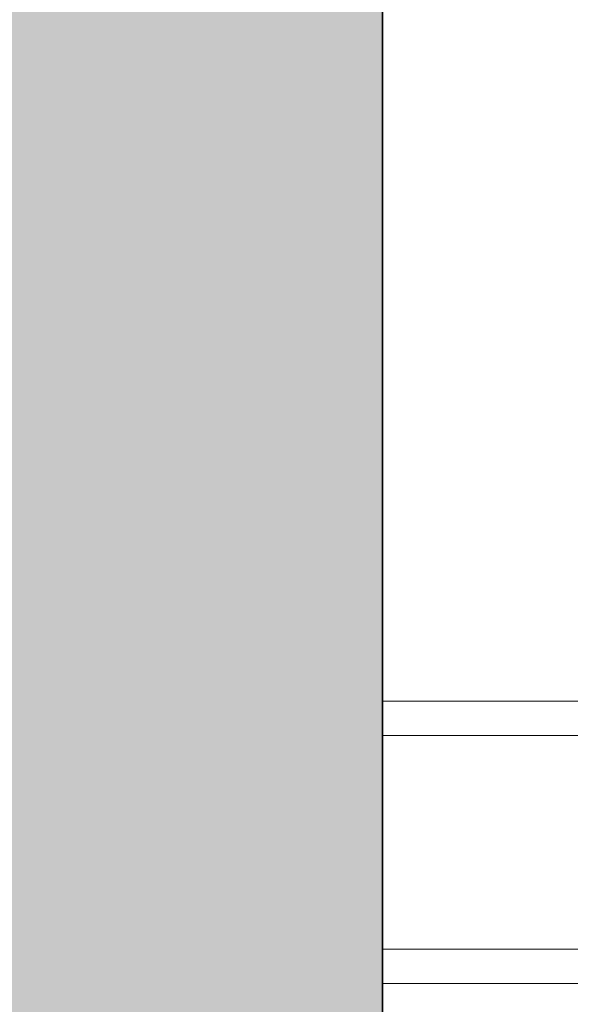
# Model space of a CAD drawing. Units: inches. Extents: x 2696 to 3240, y 1564 to 2310.
# Tile 8 of 76: x 2893.424 to 2898.411, y 1643.56 to 1652.487. Entities that reach past the tile are written whole.
import ezdxf

# ---------------------------------------------------------------- set-up
doc = ezdxf.new("R2010")
doc.units = ezdxf.units.IN
for name, color, linetype, lineweight in [('A-ANNO-DIMS', 3, 'Continuous', 18), ('A-FLOR-FIXT', 8, 'Continuous', 18), ('A-FURN', 251, 'Continuous', 13), ('A-WALL', 7, 'Continuous', 35), ('A-WALL-PATT', 9, 'Continuous', 13)]:
    doc.layers.add(name, color=color, linetype=linetype, lineweight=lineweight)
doc.layers.add('FURNITURE', color=250, linetype='Continuous')
doc.styles.add('TIMES NEW', font='times.ttf')
doc.dimstyles.new('Siddhuu', dxfattribs={"dimtxt": 6, "dimasz": 2.5, "dimexe": 1.25, "dimexo": 0.625, "dimtad": 1, "dimdec": 1, "dimlunit": 4, "dimtxsty": 'TIMES NEW', "dimcen": 2.5, "dimclrd": 256, "dimclre": 1, "dimclrt": 7, "dimadec": 0, "dimazin": 0, "dimtfac": 1, "dimtdec": 1, "dimtmove": 0, "dimatfit": 3, "dimfxl": 1, "dimtolj": 1, "dimlwd": -1, "dimarcsym": 0})

# ---------------------------------------------------------------- blocks, each defined once
blk = doc.blocks.new('A$C1af1f523')
at = {"layer": 'A-FURN'}
for p, q in [((0, 2.5605), (-4.2116, 2.5605)), ((0, 2.5605, 0.5), (-4.2116, 2.5605, 0.5)), ((0, 2.248), (-4.2116, 2.248)), ((0, 2.248, 0.5), (-4.2116, 2.248, 0.5)), ((0, 0.3125), (-6.5015, 0.3125)), ((0, 0.3125, 0.5), (-6.5015, 0.3125, 0.5)), ((0, 0), (-6.5015, 0)), ((0, 0, 0.5), (-6.5015, 0, 0.5))]:
    blk.add_line(p, q, dxfattribs=at)
at = {"layer": 'FURNITURE'}
for p, q in [((0, 2.5605), (0, 2.5605, 0.5)), ((0, 2.248), (0, 2.248, 0.5)), ((0, 0.3125), (0, 0.3125, 0.5)), ((0, 0), (0, 0, 0.5))]:
    blk.add_line(p, q, dxfattribs=at)
at = {"layer": 'A-FURN'}
mesh = blk.add_polyface(dxfattribs=at)
corners = [(0, 2.5605, 0.5), (-4.2116, 2.5605), (-4.2116, 2.5605, 0.5), (0, 2.5605)]
mesh.append_faces([[corners[k] for k in face] for face in [(2, 1, 0), (3, 0, 1)]], dxfattribs={"vtx1": -1})
mesh = blk.add_polyface(dxfattribs=at)
corners = [(0, 2.248, 0.5), (-4.2116, 2.248), (-4.2116, 2.248, 0.5), (0, 2.248)]
mesh.append_faces([[corners[k] for k in face] for face in [(2, 1, 0), (3, 0, 1)]], dxfattribs={"vtx1": -1})
mesh = blk.add_polyface(dxfattribs=at)
corners = [(0, 0.3125, 0.5), (-6.5015, 0.3125), (-6.5015, 0.3125, 0.5), (0, 0.3125)]
mesh.append_faces([[corners[k] for k in face] for face in [(2, 1, 0), (3, 0, 1)]], dxfattribs={"vtx1": -1})
mesh = blk.add_polyface(dxfattribs=at)
corners = [(0, 0, 0.5), (-6.5015, 0), (-6.5015, 0, 0.5), (0, 0)]
mesh.append_faces([[corners[k] for k in face] for face in [(2, 1, 0), (3, 0, 1)]], dxfattribs={"vtx1": -1})
blk = doc.blocks.new('*D57')
at = {"layer": 'A-ANNO-DIMS', "color": 1, "lineweight": -2, "transparency": 16777216}
for p, q in [((2754.6114, 2018.5761), (2754.6114, 1568.9511)), ((2956.7088, 2018.5761), (2956.7088, 1568.9511))]:
    blk.add_line(p, q, dxfattribs=at)
at = {"layer": 'A-ANNO-DIMS', "transparency": 16777216}
blk.add_line((2757.1114, 1570.2011), (2954.2088, 1570.2011), dxfattribs=at)
for points in [[(2757.1114, 1570.6178), (2757.1114, 1569.7844), (2754.6114, 1570.2011)], [(2954.2088, 1570.6178), (2954.2088, 1569.7844), (2956.7088, 1570.2011)]]:
    blk.add_solid(points, dxfattribs=at)
at = {"layer": 'Defpoints', "color": 0, "transparency": 16777216}
for p in [(2754.6114, 2019.2011), (2956.7088, 2019.2011), (2956.7088, 1570.2011)]:
    blk.add_point(p, dxfattribs=at)
at = {"layer": 'A-ANNO-DIMS', "color": 7, "transparency": 16777216, "insert": (2855.6601, 1573.878), "char_height": 6, "attachment_point": 5, "style": 'TIMES NEW'}
blk.add_mtext('\\A1;16\'-10"', dxfattribs=at)
blk = doc.blocks.new('*D69')
at = {"layer": 'A-ANNO-DIMS', "color": 1, "lineweight": -2, "transparency": 16777216}
for p, q in [((2841.889, 2261.5761), (2841.889, 1568.9511)), ((2905.9101, 2261.5761), (2905.9101, 1568.9511))]:
    blk.add_line(p, q, dxfattribs=at)
at = {"layer": 'A-ANNO-DIMS', "transparency": 16777216}
blk.add_line((2844.389, 1570.2011), (2903.4101, 1570.2011), dxfattribs=at)
for points in [[(2844.389, 1570.6178), (2844.389, 1569.7844), (2841.889, 1570.2011)], [(2903.4101, 1570.6178), (2903.4101, 1569.7844), (2905.9101, 1570.2011)]]:
    blk.add_solid(points, dxfattribs=at)
at = {"layer": 'Defpoints', "color": 0, "transparency": 16777216}
for p in [(2841.889, 2262.2011), (2905.9101, 2262.2011), (2905.9101, 1570.2011)]:
    blk.add_point(p, dxfattribs=at)
at = {"layer": 'A-ANNO-DIMS', "color": 7, "transparency": 16777216, "insert": (2873.8995, 1573.878), "char_height": 6, "attachment_point": 5, "style": 'TIMES NEW'}
blk.add_mtext('\\A1;5\'-4"', dxfattribs=at)

msp = doc.modelspace()

# ---------------------------------------------------------------- hatches: boundary and pattern name
at = {"layer": 'A-WALL-PATT', "transparency": 33554556}
h = msp.add_hatch(color=256, dxfattribs=at)
h.dxf.hatch_style = 1
h.paths.add_polyline_path([(2879.1114, 2253.2011), (2905.9101, 2253.2011), (2905.9101, 2262.2011), (2841.889, 2262.2011), (2841.889, 2253.2011), (2870.1114, 2253.2011), (2870.1114, 2176.6011), (2965.7088, 2176.6011), (2965.7088, 2206.7011), (2973.5828, 2206.7011), (2973.5828, 2215.7011), (2965.7088, 2215.7011), (2965.7088, 2262.2011), (2929.9101, 2262.2011), (2929.9101, 2253.2011), (2956.7088, 2253.2011), (2956.7088, 2185.6011), (2879.1114, 2185.6011)])
h.paths.add_polyline_path([(2782.8338, 2262.2011), (2745.6114, 2262.2011), (2745.6114, 2228.7287), (2754.6114, 2228.7287), (2754.6114, 2253.2011), (2782.8338, 2253.2011)])
h.paths.add_polyline_path([(2754.6114, 2136.2011), (2965.7088, 2136.2011), (2965.7088, 2145.2011), (2879.1114, 2145.2011), (2879.1114, 2147.0735), (2877.3397, 2147.0735), (2870.1114, 2147.0735), (2870.1114, 2145.2011), (2754.6114, 2145.2011), (2754.6114, 2169.6735), (2745.6114, 2169.6735), (2745.6114, 2000.2011), (2754.6114, 2000.2011), (2754.6114, 2019.2011), (2849.0828, 2019.2011), (2849.0828, 2023.7011), (2841.2088, 2023.7011), (2841.2088, 2051.8271), (2836.7088, 2051.8271), (2836.7088, 2023.7011), (2754.6114, 2023.7011), (2754.6114, 2091.2011), (2836.7088, 2091.2011), (2836.7088, 2087.8271), (2841.2088, 2087.8271), (2841.2088, 2095.7011), (2754.6114, 2095.7011)])
h.paths.add_polyline_path([(2965.7088, 2136.2011), (2956.7088, 2136.2011), (2956.7088, 2023.7011), (2885.0828, 2023.7011), (2885.0828, 2019.2011), (2956.7088, 2019.2011), (2956.7088, 1950.5751), (2965.7088, 1950.5751), (2965.7088, 1980.2011), (2973.5828, 1980.2011), (2973.5828, 1989.2011), (2965.7088, 1989.2011)])
h.paths.add_polyline_path([(2754.6114, 1906.7011), (2880.2088, 1906.7011), (2884.7088, 1906.7011), (2956.7088, 1906.7011), (2956.7088, 1792.7011), (2944.7088, 1792.7011), (2944.7088, 1783.7011), (2956.7088, 1783.7011), (2956.7088, 1740.2011), (2884.7088, 1740.2011), (2884.7088, 1783.7011), (2896.7088, 1783.7011), (2896.7088, 1792.7011), (2884.7088, 1792.7011), (2884.7088, 1846.7011), (2880.2088, 1846.7011), (2880.2088, 1740.2011), (2754.6114, 1740.2011), (2754.6114, 1777.2011), (2745.6114, 1777.2011), (2745.6114, 1692.7011), (2754.6114, 1692.7011), (2754.6114, 1731.2011), (2956.7088, 1731.2011), (2956.7088, 1723.3271), (2965.7088, 1723.3271), (2965.7088, 1884.2011), (2973.5828, 1884.2011), (2973.5828, 1893.2011), (2965.7088, 1893.2011), (2965.7088, 1914.5751), (2956.7088, 1914.5751), (2956.7088, 1911.2011), (2754.6114, 1911.2011), (2754.6114, 1930.2011), (2745.6114, 1930.2011), (2745.6114, 1817.2011), (2754.6114, 1817.2011), (2754.6114, 1854.2011), (2826.6114, 1854.2011), (2826.6114, 1868.8271), (2822.1114, 1868.8271), (2822.1114, 1858.7011), (2754.6114, 1858.7011)])
h.paths.add_polyline_path([(2965.7088, 1656.2011), (3008.2374, 1656.2011), (3008.2374, 1665.2011), (2965.7088, 1665.2011), (2965.7088, 1693.3271), (2956.7088, 1693.3271), (2956.7088, 1686.2011), (2934.5828, 1686.2011), (2934.5828, 1681.7011), (2956.7088, 1681.7011), (2956.7088, 1614.2011), (2896.7088, 1614.2011), (2896.7088, 1681.7011), (2904.5828, 1681.7011), (2904.5828, 1686.2011), (2892.2088, 1686.2011), (2892.2088, 1614.2011), (2858.4101, 1614.2011), (2858.4101, 1605.2011), (2965.7088, 1605.2011)])
h.paths.add_polyline_path([(2788.4101, 1614.2011), (2754.6114, 1614.2011), (2754.6114, 1652.7011), (2745.6114, 1652.7011), (2745.6114, 1605.2011), (2788.4101, 1605.2011)])
h.paths.add_polyline_path([(3199.6114, 1633.0476), (3190.6114, 1633.0476), (3190.6114, 1614.2011), (3082.6114, 1614.2011), (3082.6114, 1665.2011), (3070.2374, 1665.2011), (3070.2374, 1656.2011), (3078.1114, 1656.2011), (3078.1114, 1605.2011), (3199.6114, 1605.2011)])
h.paths.add_polyline_path([(3199.6114, 1702.0476), (3190.6114, 1702.0476), (3190.6114, 1699.7011), (3106.6114, 1699.7011), (3106.6114, 1747.7011), (3190.6114, 1747.7011), (3190.6114, 1752.2011), (3082.6114, 1752.2011), (3082.6114, 1760.0751), (3078.1114, 1760.0751), (3078.1114, 1747.7011), (3102.1114, 1747.7011), (3102.1114, 1699.7011), (3078.1114, 1699.7011), (3078.1114, 1695.2011), (3190.6114, 1695.2011), (3190.6114, 1676.3546), (3199.6114, 1676.3546)])
h.paths.add_polyline_path([(3199.6114, 1783.2011), (3190.6114, 1783.2011), (3190.6114, 1745.3546), (3199.6114, 1745.3546)])
h.paths.add_polyline_path([(3082.6114, 1884.2011), (3190.6114, 1884.2011), (3190.6114, 1853.2011), (3199.6114, 1853.2011), (3199.6114, 1901.7011), (3190.6114, 1901.7011), (3190.6114, 1893.2011), (3005.5828, 1893.2011), (3005.5828, 1891.2811), (3005.5828, 1884.2011), (3078.1114, 1884.2011), (3078.1114, 1792.0751), (3082.6114, 1792.0751)])
h.paths.add_polyline_path([(3199.6114, 1994.7011), (3190.6114, 1994.7011), (3190.6114, 1989.2011), (3073.7088, 1989.2011), (3073.7088, 2034.2011), (3069.2088, 2034.2011), (3069.2088, 1989.2011), (3005.5828, 1989.2011), (3005.5828, 1980.2011), (3190.6114, 1980.2011), (3190.6114, 1971.7011), (3199.6114, 1971.7011)])
h.paths.add_polyline_path([(3199.6114, 2155.2011), (3190.6114, 2155.2011), (3190.6114, 2064.7011), (3199.6114, 2064.7011)])
h.paths.add_polyline_path([(3190.6114, 2074.7011), (3106.6114, 2074.7011), (3106.6114, 2122.7011), (3190.6114, 2122.7011), (3190.6114, 2127.2011), (3082.7088, 2127.2011), (3082.7088, 2135.0751), (3073.7088, 2135.0751), (3073.7088, 2122.7011), (3102.1114, 2122.7011), (3102.1114, 2074.7011), (3069.2088, 2074.7011), (3069.2088, 2070.2011), (3190.6114, 2070.2011)])
h.paths.add_polyline_path([(3082.7088, 2253.2011), (3190.6114, 2253.2011), (3190.6114, 2225.2011), (3199.6114, 2225.2011), (3199.6114, 2262.2011), (3073.7088, 2262.2011), (3073.7088, 2215.7011), (3035.5828, 2215.7011), (3035.5828, 2206.7011), (3073.7088, 2206.7011), (3073.7088, 2171.0751), (3082.7088, 2171.0751)])

# ---------------------------------------------------------------- linework, layer by layer
at = {"layer": 'A-WALL'}
msp.add_line((2896.7088, 1681.7011), (2896.7088, 1614.2011), dxfattribs=at)

# ---------------------------------------------------------------- block references
at = {"layer": 'A-FLOR-FIXT', "xscale": -1}
msp.add_blockref('A$C1af1f523', (2896.7088, 1643.7478), dxfattribs=at)

# ---------------------------------------------------------------- dimensions: what is measured, and where the dimension line sits
at = {"layer": 'A-ANNO-DIMS'}
for base, p1, p2, picture, middle in [((2905.9101, 1570.2011), (2841.889, 2262.2011), (2905.9101, 2262.2011), '*D69', (2873.8995, 1573.878)), ((2956.7088, 1570.2011), (2754.6114, 2019.2011), (2956.7088, 2019.2011), '*D57', (2855.6601, 1573.878))]:
    dim = msp.add_linear_dim(base=base, p1=p1, p2=p2, dimstyle='Siddhuu', override={"dimdec": 1, "dimlfac": 1, "dimrnd": 0, "dimzin": 1, "dimdsep": 46, "dimlunit": 4, "dimfrac": 2}, dxfattribs=at)
    dim.commit()
    dim.dimension.update_dxf_attribs({"geometry": picture, "text_midpoint": middle})

doc.saveas('drawing.dxf')
